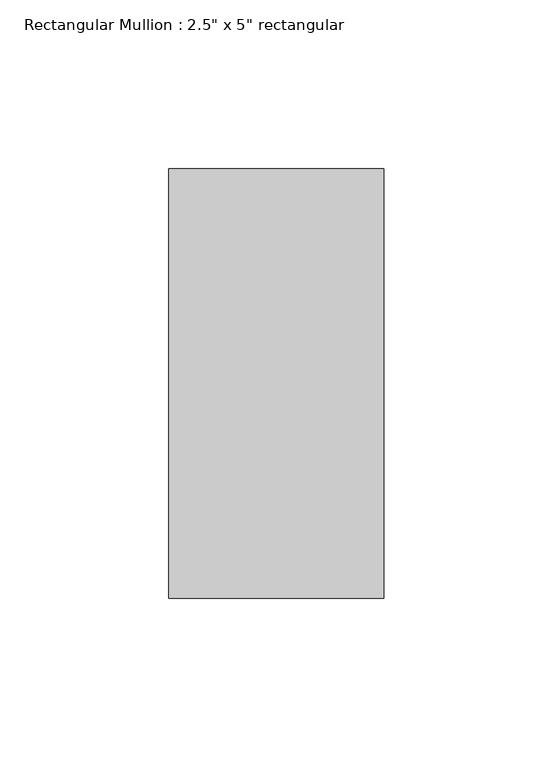
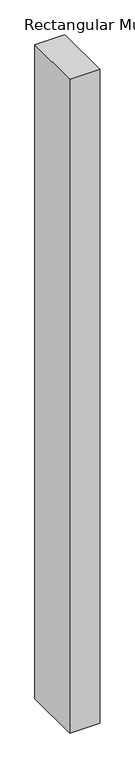
"""IFC4 building model written with IfcOpenShell, lengths in millimetres: member geometry."""

from ifc_helpers import new_model, si_unit, frame, origin, place, context, project, spatial, polyline, outline, extrude, source, transform, mapped, element, save


def member_4a1dde21(model_context):
    return source(origin(), model_context, "Body", "SweptSolid", [
        extrude(outline(polyline([(0.0, 63.5), (0.0, -63.5), (-63.5, -63.5), (-63.5, 63.5), (0.0, 63.5)])), frame((0.0, 0.0, -1460.5), z_axis=(0.0, 0.0, 1.0), x_axis=(1.0, 0.0, 0.0)), (0.0, 0.0, 1.0), 1460.5),
    ])


if __name__ == "__main__":
    model = new_model("IFC4")
    model_context = context("Model", 3, world=origin())
    ifc_project = project(units=[si_unit("LENGTHUNIT", "METRE", prefix="MILLI")], contexts=[model_context])
    site = spatial("IfcSite", under=ifc_project)
    building = spatial("IfcBuilding", under=site)
    placement = place(None, origin())
    member_shape = member_4a1dde21(model_context)
    element("IfcMember", 1, ObjectType="Rectangular Mullion : 2.5\" x 5\" rectangular", at=placement, inside=building, context=model_context, shape_type="MappedRepresentation", body=[
        mapped(member_shape, transform((0.0, 0.0, 0.0), x_axis=(1.0, 0.0, 0.0), y_axis=(0.0, 1.0, 0.0), z_axis=(0.0, 0.0, 1.0))),
    ])
    save(model, "model.ifc")

# Revit data of these elements
# Type "Rectangular Mullion : 2.5\" x 5\" rectangular"
#   built-in parameter 1007304 = 0.416667 (stored number, unit not read)
#   built-in parameter 1007301 = 0.104167 (stored number, unit not read)
#   built-in parameter 1007300 = 0.104167 (stored number, unit not read)
# Element 1 (IfcMember, "Rectangular Mullion : 2.5\" x 5\" rectangular")
#   Materials on its faces: "Aluminum"
# Materials
#   "Aluminum": class "Metal", colour RGB 247 247 247, transparency 0, Description = "Aluminum 6061", Cost = 0
